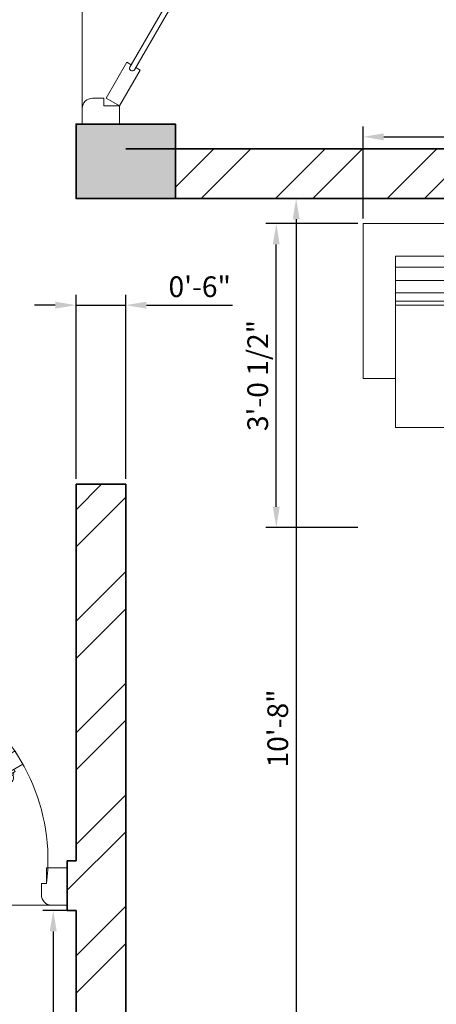
# Model space of a CAD drawing. Units: inches. Extents: x -138 to 270, y 8284 to 8764.
# Tile 6 of 10: x 61 to 112, y 8387 to 8506. Entities that reach past the tile are written whole.
import ezdxf

# ---------------------------------------------------------------- set-up
doc = ezdxf.new("R2010")
doc.units = ezdxf.units.IN
for name, color, linetype, lineweight in [('A-ANNO-DIMS', 2, 'Continuous', 18), ('DOOR', 32, 'Continuous', 15), ('FURNITURE', 8, 'Continuous', 15), ('FURNITURE1', 8, 'Continuous', 15), ('WALL', 8, 'Continuous', 35)]:
    doc.layers.add(name, color=color, linetype=linetype, lineweight=lineweight)
doc.layers.add('A-COLS', color=252, linetype='Continuous', lineweight=35, true_color=0x939598)
doc.layers.add('A-WALL-PATT', color=32, linetype='Continuous', lineweight=9, true_color=0xbc761a)
doc.styles.get("Standard").update_dxf_attribs({"font": 'arial.ttf'})
doc.dimstyles.new('ISO-25', dxfattribs={"dimtxt": 2.5, "dimasz": 2.5, "dimexe": 1.25, "dimexo": 0.625, "dimtad": 1, "dimdec": 0, "dimlunit": 3, "dimtxsty": 'Standard', "dimcen": 2.5, "dimadec": 0, "dimazin": 0, "dimtfac": 1, "dimtdec": 0, "dimtmove": 0, "dimatfit": 3, "dimfxl": 1, "dimarcsym": 0})

# ---------------------------------------------------------------- blocks, each defined once
blk = doc.blocks.new('A$C1A8229D7')
at = {"layer": 'DOOR'}
for p, q in [((22.38, 16.16), (26.71, 18.66)), ((24.39, 17.68), (25.47, 18.3)), ((24.56, 18), (25.1, 18.31)), ((24.56, 18), (24.66, 17.83)), ((24.56, 18), (24.56, 18)), ((24.83, 18.15), (24.83, 18.15)), ((25.1, 18.31), (25.2, 18.15)), ((25.47, 18.3), (25.62, 18.03)), ((27.64, 17.03), (26.71, 18.66)), ((23.31, 14.53), (27.64, 17.03)), ((24.39, 17.68), (24.54, 17.41)), ((6.56, 6.3), (22.96, 15.77)), ((22.69, 15.61), (22.38, 16.16)), ((23.39, 15.66), (23.39, 15.66)), ((25.64, 15.51), (25.48, 15.78)), ((25.64, 15.51), (26.72, 16.14)), ((26, 15.51), (25.91, 15.67)), ((26, 15.51), (26.54, 15.82)), ((26, 15.51), (26, 15.51)), ((26.27, 15.66), (26.27, 15.66)), ((26.54, 15.82), (26.45, 15.98)), ((26.72, 16.14), (26.56, 16.41)), ((23.27, 15.23), (6.87, 5.76)), ((7.14, 5.92), (23, 15.07)), ((23.31, 14.53), (23, 15.07)), ((6.52, 7), (2.19, 4.5)), ((6.83, 6.46), (6.52, 7)), ((7.46, 5.38), (3.12, 2.88)), ((6.45, 5.88), (6.45, 5.88)), ((7.46, 5.38), (7.14, 5.92)), ((0, 0), (0, 4.5)), ((0, 4.5), (2.19, 4.5)), ((2.19, 2.62), (2.19, 4.5)), ((3.12, 2.88), (2.19, 4.5)), ((30.5, 2.62), (30.5, 4.5)), ((33, 4.5), (30.5, 4.5)), ((33, 0), (33, 4.5)), ((2.19, 2.62), (3.12, 2.62)), ((3.12, 1.25), (3.12, 2.62)), ((29.87, 1.25), (29.87, 2.62)), ((30.5, 2.62), (29.87, 2.62)), ((0, 0), (1.87, 0)), ((33, 0), (0, 0)), ((0, 0), (33, 0)), ((33, 0), (31.12, 0))]:
    blk.add_line(p, q, dxfattribs=at)
at = {"layer": 'DOOR', "ltscale": 0.1}
blk.add_arc((6.98, 5.45), 23.69, 353.1504, 56.0415, dxfattribs=at)
at = {"layer": 'DOOR'}
for centre, radius, start, end in [((25.46, 15.13), 3.63, 111.4546, 145.7774), ((27.78, 10.32), 8.61, 114.2033, 127.709), ((24.4, 17.99), 0.592, 22.7059, 117.5689), ((24.41, 17.91), 0.312, 30, 120), ((22.48, 17.15), 0.0372, 138.2373, 332.5518), ((23.12, 15.5), 0.312, 30, 120), ((23.12, 15.5), 0.312, 300, 30), ((25.85, 15.42), 0.312, 300, 30), ((25.92, 15.37), 0.592, 302.4311, 37.2941), ((20.96, 22.13), 8.61, 292.291, 305.7967), ((23.97, 17.71), 3.63, 274.2226, 308.5454), ((24.23, 14.13), 0.0372, 87.4482, 281.7627), ((6.72, 6.03), 0.312, 120, 210), ((6.72, 6.03), 0.312, 210, 300), ((1.87, 1.25), 1.25, 270, 0), ((31.12, 1.25), 1.25, 180, 270)]:
    blk.add_arc(centre, radius, start, end, dxfattribs=at)
blk = doc.blocks.new('A$C48A43CE3')
at = {"layer": 'FURNITURE1'}
for points in [[(76.57, 20.9), (81.14, 20.9), (81.14, 42.62), (0, 42.62), (0, 20.9), (4.57, 20.9)], [(61.35, 14.04), (4.57, 14.04), (4.57, 38.04), (76.57, 38.04), (76.57, 30.12)], [(4.57, 14.04), (4.57, 38.04)], [(76.57, 36.51), (4.57, 36.51)], [(21.78, 34.62), (4.57, 34.62)], [(13.35, 32.9), (4.57, 32.9)], [(13.07, 31.76), (4.57, 31.76)], [(12.99, 31.19), (4.57, 31.19)]]:
    blk.add_lwpolyline(points, dxfattribs=at)
blk = doc.blocks.new('*D22')
at = {"layer": 'A-ANNO-DIMS', "color": 0, "lineweight": -2, "transparency": 16777216}
for p, q in [((94.04, 8484.24), (93.42, 8484.24)), ((94.67, 8481.74), (94.67, 8358.74)), ((94.04, 8356.24), (93.42, 8356.24))]:
    blk.add_line(p, q, dxfattribs=at)
at = {"layer": 'A-ANNO-DIMS', "color": 0, "transparency": 16777216}
for points in [[(94.25, 8481.74), (95.09, 8481.74), (94.67, 8484.24)], [(94.25, 8358.74), (95.09, 8358.74), (94.67, 8356.24)]]:
    blk.add_solid(points, dxfattribs=at)
at = {"layer": 'Defpoints', "color": 0, "transparency": 16777216}
for p in [(94.67, 8484.24), (94.67, 8356.24), (94.67, 8356.24)]:
    blk.add_point(p, dxfattribs=at)
at = {"layer": 'A-ANNO-DIMS', "color": 0, "transparency": 16777216, "insert": (92.77, 8420.24), "char_height": 2.5, "attachment_point": 5, "rotation": 90}
blk.add_mtext('10\'-8"', dxfattribs=at)
blk = doc.blocks.new('*D25')
at = {"layer": 'A-ANNO-DIMS', "color": 0, "lineweight": -2, "transparency": 16777216}
for p, q in [((67.45, 8398.24), (64.08, 8398.24)), ((65.33, 8395.74), (65.33, 8358.74)), ((67.45, 8356.24), (64.08, 8356.24))]:
    blk.add_line(p, q, dxfattribs=at)
at = {"layer": 'A-ANNO-DIMS', "color": 0, "transparency": 16777216}
for points in [[(64.91, 8395.74), (65.75, 8395.74), (65.33, 8398.24)], [(64.91, 8358.74), (65.75, 8358.74), (65.33, 8356.24)]]:
    blk.add_solid(points, dxfattribs=at)
at = {"layer": 'Defpoints', "color": 0, "transparency": 16777216}
for p in [(68.08, 8398.24), (65.33, 8356.24), (68.08, 8356.24)]:
    blk.add_point(p, dxfattribs=at)
at = {"layer": 'A-ANNO-DIMS', "color": 0, "transparency": 16777216, "insert": (63.43, 8377.24), "char_height": 2.5, "attachment_point": 5, "rotation": 90}
blk.add_mtext('3\'-6"', dxfattribs=at)
blk = doc.blocks.new('COLUMN-9X12IN')
h = blk.add_hatch(color=256)
h.dxf.hatch_style = 1
h.paths.add_polyline_path([(9, 12), (0, 12), (0, 0), (9, 0)])
blk.add_lwpolyline([(0, 0), (9, 0), (9, 12), (0, 12)], close=True)
blk = doc.blocks.new('*D41')
at = {"layer": 'A-ANNO-DIMS', "color": 0, "lineweight": -2, "transparency": 16777216}
for p, q in [((102.75, 8481.84), (102.75, 8492.95)), ((172.62, 8481.84), (172.62, 8492.95)), ((105.25, 8491.7), (170.12, 8491.7))]:
    blk.add_line(p, q, dxfattribs=at)
at = {"layer": 'A-ANNO-DIMS', "color": 0, "transparency": 16777216}
for points in [[(105.25, 8492.11), (105.25, 8491.28), (102.75, 8491.7)], [(170.12, 8492.11), (170.12, 8491.28), (172.62, 8491.7)]]:
    blk.add_solid(points, dxfattribs=at)
at = {"layer": 'Defpoints', "color": 0, "transparency": 16777216}
for p in [(172.62, 8491.7), (102.75, 8481.21), (172.62, 8481.21)]:
    blk.add_point(p, dxfattribs=at)
at = {"layer": 'A-ANNO-DIMS', "color": 0, "transparency": 16777216, "insert": (137.69, 8493.61), "char_height": 2.5, "attachment_point": 5}
blk.add_mtext('SOFA 5\'-10"', dxfattribs=at)
blk = doc.blocks.new('*D42')
at = {"layer": 'A-ANNO-DIMS', "color": 0, "lineweight": -2, "transparency": 16777216}
for p, q in [((102.12, 8481.21), (91.02, 8481.21)), ((92.27, 8447.02), (92.27, 8478.71)), ((102.12, 8444.52), (91.02, 8444.52))]:
    blk.add_line(p, q, dxfattribs=at)
at = {"layer": 'A-ANNO-DIMS', "color": 0, "transparency": 16777216}
for points in [[(91.85, 8478.71), (92.68, 8478.71), (92.27, 8481.21)], [(91.85, 8447.02), (92.68, 8447.02), (92.27, 8444.52)]]:
    blk.add_solid(points, dxfattribs=at)
at = {"layer": 'Defpoints', "color": 0, "transparency": 16777216}
for p in [(92.27, 8481.21), (102.75, 8481.21), (102.75, 8444.52)]:
    blk.add_point(p, dxfattribs=at)
at = {"layer": 'A-ANNO-DIMS', "color": 0, "transparency": 16777216, "insert": (90.35, 8462.87), "char_height": 2.5, "attachment_point": 5, "rotation": 90}
blk.add_mtext('3\'-0 1/2"', dxfattribs=at)
blk = doc.blocks.new('*D76')
at = {"layer": 'A-ANNO-DIMS', "color": 0, "lineweight": -2, "transparency": 16777216}
for p, q in [((68.08, 8450.38), (68.08, 8472.62)), ((74.08, 8450.38), (74.08, 8472.62)), ((65.58, 8471.37), (63.08, 8471.37)), ((68.08, 8471.37), (74.08, 8471.37)), ((76.58, 8471.37), (86.97, 8471.37))]:
    blk.add_line(p, q, dxfattribs=at)
at = {"layer": 'A-ANNO-DIMS', "color": 0, "transparency": 16777216}
for points in [[(65.58, 8471.78), (65.58, 8470.95), (68.08, 8471.37)], [(76.58, 8471.78), (76.58, 8470.95), (74.08, 8471.37)]]:
    blk.add_solid(points, dxfattribs=at)
at = {"layer": 'Defpoints', "color": 0, "transparency": 16777216}
for p in [(74.08, 8471.37), (68.08, 8449.75), (74.08, 8449.75)]:
    blk.add_point(p, dxfattribs=at)
at = {"layer": 'A-ANNO-DIMS', "color": 0, "transparency": 16777216, "insert": (83.02, 8473.27), "char_height": 2.5, "attachment_point": 5}
blk.add_mtext('0\'-6"', dxfattribs=at)

msp = doc.modelspace()

# ---------------------------------------------------------------- hatches: boundary and pattern name
at = {"layer": 'A-WALL-PATT'}
h = msp.add_hatch(dxfattribs=at)
h.set_pattern_fill('ANSI32', color=256)
h.paths.add_polyline_path([(115.81, 8699.24), (65.22, 8699.24), (65.22, 8690.24), (68.08, 8690.24), (68.08, 8686.36), (69.02, 8686.36), (69.02, 8686.36), (73.52, 8686.36), (74.08, 8686.36), (74.08, 8690.24), (115.81, 8690.24)])
h.paths.add_polyline_path([(169.81, 8699.24), (139.81, 8699.24), (139.81, 8690.24), (169.81, 8690.24)])
h.paths.add_polyline_path([(198.08, 8699.24), (193.81, 8699.24), (193.81, 8690.24), (198.08, 8690.24)])
h.paths.add_polyline_path([(207.08, 8648.24), (204.23, 8648.24), (204.23, 8648.24), (199.73, 8648.24), (198.08, 8648.24), (198.08, 8642.24), (150.08, 8642.24), (150.08, 8690.24), (144.08, 8690.24), (144.08, 8642.24), (74.08, 8642.24), (74.08, 8653.36), (68.08, 8653.36), (68.08, 8526.24), (68.83, 8526.24), (74.08, 8526.24), (74.08, 8630.24), (74.08, 8636.24), (98.08, 8636.24), (150.08, 8636.24), (198.08, 8636.24), (198.08, 8630.24), (198.08, 8532.24), (207.08, 8532.24)])
h.paths.add_polyline_path([(207.08, 8484.24), (198.08, 8484.24), (198.08, 8433.43), (207.08, 8433.43)])
h.paths.add_polyline_path([(198.08, 8490.24), (80.08, 8490.24), (80.08, 8484.24), (198.08, 8484.24)])
h.paths.add_polyline_path([(207.08, 8397.43), (198.08, 8397.43), (198.08, 8359.27), (207.08, 8359.27)])
h.paths.add_polyline_path([(198.08, 8356.24), (186.08, 8356.24), (186.08, 8347.24), (198.08, 8347.24)])
h.paths.add_polyline_path([(138.08, 8356.24), (128.38, 8356.24), (128.38, 8347.24), (138.08, 8347.24)])
h.paths.add_polyline_path([(92.38, 8356.24), (86.08, 8356.24), (86.08, 8347.24), (92.38, 8347.24)])
h = msp.add_hatch(dxfattribs=at)
h.set_pattern_fill('ANSI32', color=256)
h.paths.add_polyline_path([(-23.4, 8356.24), (-63.92, 8356.24), (-63.92, 8347.24), (-23.4, 8347.24)])
h.paths.add_polyline_path([(-63.92, 8469.84), (-72.92, 8469.84), (-72.92, 8359.24), (-63.92, 8359.24)])
h.paths.add_polyline_path([(-63.92, 8510.27), (-72.92, 8510.27), (-72.92, 8505.84), (-63.92, 8505.84)])
h.paths.add_polyline_path([(-63.92, 8527.36), (-72.92, 8527.36), (-72.92, 8522.27), (-63.92, 8522.27)])
h.paths.add_polyline_path([(26.08, 8522.24), (24.78, 8522.24), (24.78, 8522.24), (20.08, 8522.24), (20.08, 8516.24), (-63.92, 8516.24), (-63.92, 8510.24), (26.08, 8510.24)])
h.paths.add_polyline_path([(34.02, 8398.24), (34.02, 8404.24), (26.08, 8404.24), (26.08, 8356.24), (12.6, 8356.24), (12.6, 8347.24), (37.77, 8347.24), (37.77, 8356.24), (32.08, 8356.24), (32.08, 8398.24)])
h.paths.add_polyline_path([(67.02, 8404.24), (67.02, 8398.24), (68.08, 8398.24), (68.08, 8356.24), (61.77, 8356.24), (61.77, 8347.24), (74.08, 8347.24), (74.08, 8356.24), (74.08, 8356.24), (74.08, 8449.75), (68.08, 8449.75), (68.08, 8404.24)])

# ---------------------------------------------------------------- linework, layer by layer
at = {"layer": 'WALL'}
for p, q in [((74.08, 8493.24), (68.08, 8493.24)), ((74.08, 8490.24), (198.08, 8490.24)), ((74.08, 8484.24), (198.08, 8484.24)), ((74.08, 8484.24), (74.08, 8484.24)), ((68.08, 8449.75), (68.08, 8404.24)), ((74.08, 8449.75), (68.08, 8449.75)), ((74.08, 8449.75), (74.08, 8356.24)), ((67.02, 8404.24), (67.02, 8398.24)), ((67.02, 8404.24), (68.08, 8404.24)), ((67.02, 8398.24), (68.08, 8398.24)), ((68.08, 8398.24), (68.08, 8356.24))]:
    msp.add_line(p, q, dxfattribs=at)

# ---------------------------------------------------------------- block references
at = {"layer": 'A-COLS', "rotation": 89.999999999989}
msp.add_blockref('COLUMN-9X12IN', (80.08, 8484.24), dxfattribs=at)
at = {"layer": 'DOOR', "xscale": -1, "rotation": 270}
msp.add_blockref('A$C1A8229D7', (68.83, 8493.24), dxfattribs=at)
at = {"layer": 'DOOR'}
msp.add_blockref('A$C1A8229D7', (34.02, 8398.9), dxfattribs=at)
at = {"layer": 'FURNITURE', "xscale": 0.8611257712950477, "yscale": 0.8611257712950477, "zscale": 0.8611257712950477}
msp.add_blockref('A$C48A43CE3', (102.75, 8444.52), dxfattribs=at)

# ---------------------------------------------------------------- dimensions: what is measured, and where the dimension line sits
at = {"layer": 'A-ANNO-DIMS'}
dim = msp.add_linear_dim(base=(172.62, 8491.7), p1=(102.75, 8481.21), p2=(172.62, 8481.21), text='SOFA <>', dimstyle='ISO-25', override={"dimdec": 1, "dimlfac": 1, "dimrnd": 0, "dimzin": 1, "dimdsep": 46, "dimlunit": 4, "dimfrac": 2}, dxfattribs=at)
dim.commit()
dim.dimension.update_dxf_attribs({"geometry": '*D41', "text_midpoint": (137.69, 8493.61)})
for p1, p2, distance, picture, middle in [((94.67, 8484.24), (94.67, 8356.24), 0, '*D22', (92.77, 8420.24)), ((68.08, 8398.24), (68.08, 8356.24), -2.75, '*D25', (63.43, 8377.24))]:
    dim = msp.add_aligned_dim(p1=p1, p2=p2, distance=distance, dimstyle='ISO-25', override={"dimclrd": 0, "dimclre": 0, "dimclrt": 0}, dxfattribs=at)
    dim.commit()
    dim.dimension.update_dxf_attribs({"geometry": picture, "text_midpoint": middle})
dim = msp.add_linear_dim(base=(92.27, 8481.21), p1=(102.75, 8444.52), p2=(102.75, 8481.21), angle=90, dimstyle='ISO-25', override={"dimdec": 1, "dimlfac": 1, "dimrnd": 0, "dimzin": 1, "dimdsep": 46, "dimlunit": 4, "dimfrac": 2}, dxfattribs=at)
dim.commit()
dim.dimension.update_dxf_attribs({"geometry": '*D42', "text_midpoint": (90.35, 8462.87)})
dim = msp.add_linear_dim(base=(74.08, 8471.37), p1=(68.08, 8449.75), p2=(74.08, 8449.75), dimstyle='ISO-25', override={"dimdec": 1, "dimlfac": 1, "dimrnd": 0, "dimzin": 1, "dimdsep": 46, "dimlunit": 4, "dimfrac": 2}, dxfattribs=at)
dim.commit()
dim.dimension.update_dxf_attribs({"geometry": '*D76', "text_midpoint": (83.02, 8473.27)})

doc.saveas('drawing.dxf')
